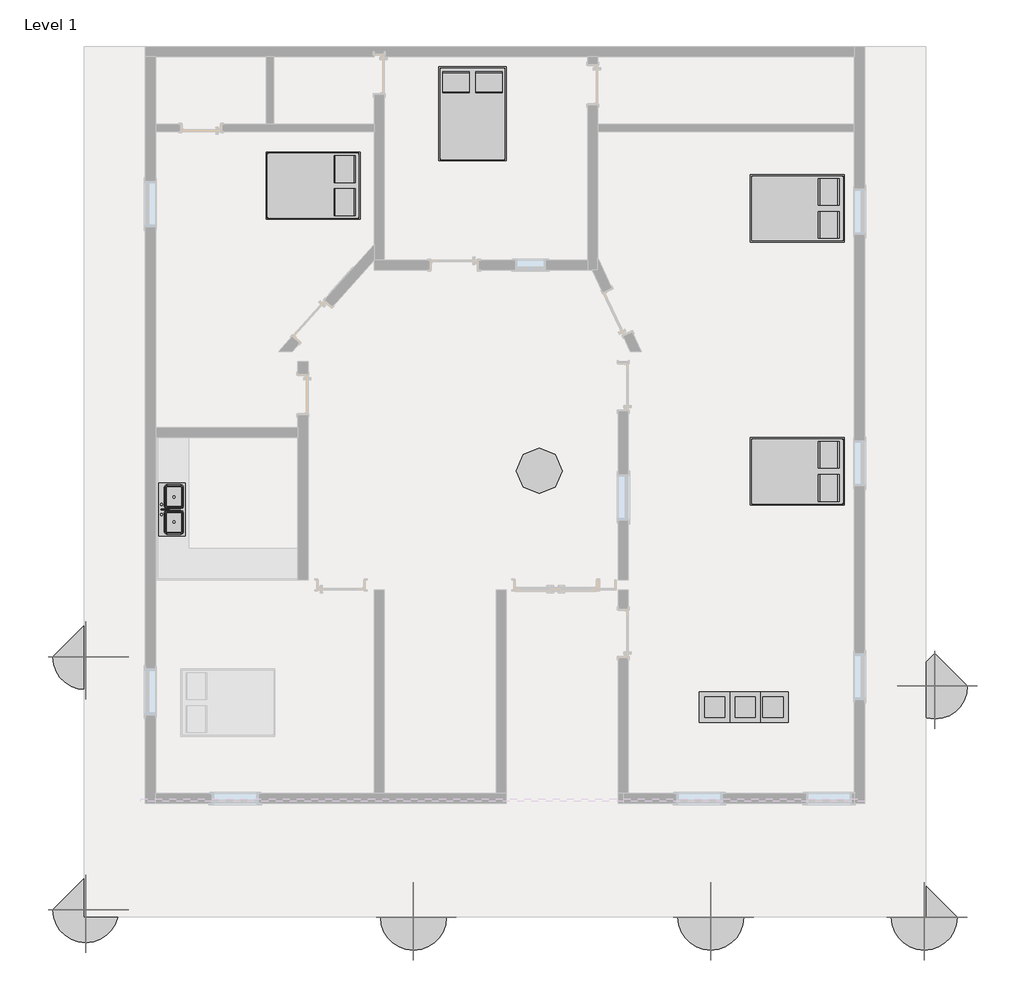
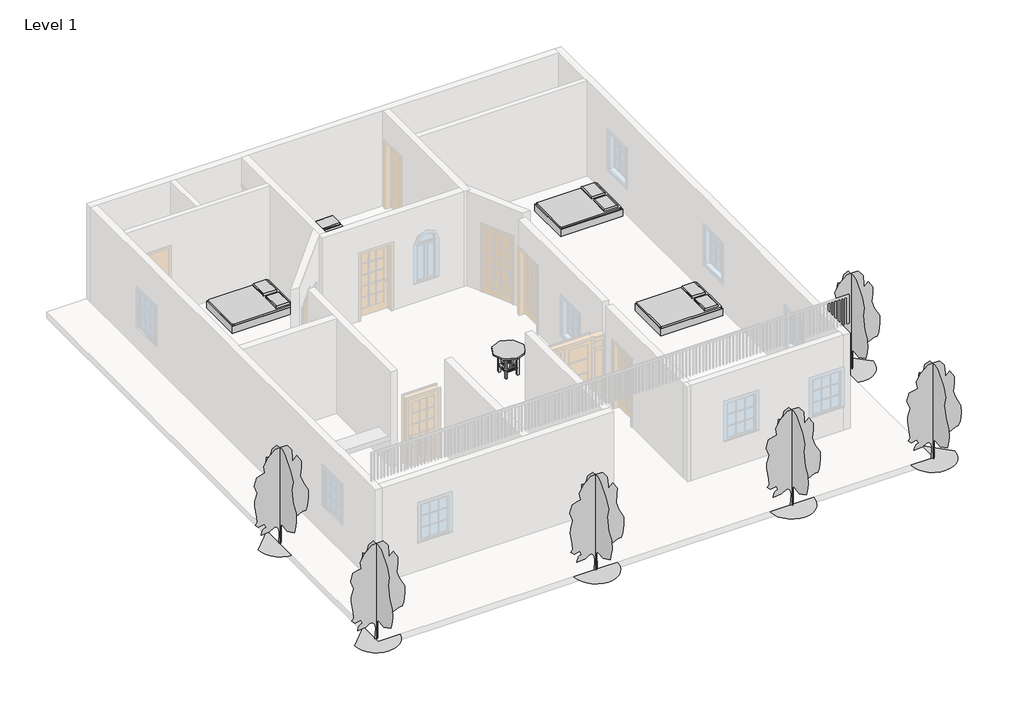
# One storey, part 3 of 3: 8 furniture elements, 6 geographic elements, 1 flow terminal.
"""IFC4 building model written with IfcOpenShell, lengths in millimetres."""

from ifc_helpers import new_model, si_unit, origin, place, context, project, spatial, transform, mapped, element, save
from components import flow_terminal_a53be723, furniture_c8abb964, furniture_b5c51a22, furniture_905aceb5, rpc_tree_deciduous_red_ash_25_5dd3353f

model = new_model("IFC4")

# Units and contexts
model_context = context("Model", 3, world=origin())
ifc_project = project(units=[si_unit("LENGTHUNIT", "METRE", prefix="MILLI")], contexts=[model_context])

# Site, building, storey
site = spatial("IfcSite", under=ifc_project)
building = spatial("IfcBuilding", under=site)
storey = spatial("IfcBuildingStorey", under=building, Name="Level 1", Elevation=0.0)

# Flow terminal
placement = place(None, origin())
flow_terminal_shape = flow_terminal_a53be723(model_context)
element("IfcFlowTerminal", 1, ObjectType="Sink Kitchen-Double : 42\" x 21\"", at=placement, inside=storey, context=model_context, shape_type="MappedRepresentation", body=[
    mapped(flow_terminal_shape, transform((-9002.3643866, 9259.041554, 0.0), x_axis=(0.0, 1.0, 0.0), y_axis=(-1.0, 0.0, 0.0), z_axis=(0.0, 0.0, 1.0))),
])

# Furniture
furniture_shape = furniture_c8abb964(model_context)
element("IfcFurniture", 2, ObjectType="Bed-Box : Double 53\" x 74\"", at=placement, inside=storey, context=model_context, shape_type="MappedRepresentation", body=[
    mapped(furniture_shape, transform((-3336.7622467, 17421.2603028, 0.0), x_axis=(1.0, 0.0, 0.0), y_axis=(0.0, 1.0, 0.0), z_axis=(0.0, 0.0, 1.0))),
])
element("IfcFurniture", 3, ObjectType="Bed-Box : Double 53\" x 74\"", at=placement, inside=storey, context=model_context, shape_type="MappedRepresentation", body=[
    mapped(furniture_shape, transform((-5950.8802795, 16090.8832536, 0.0), x_axis=(0.0, -0.9999999999999997, 0.0), y_axis=(0.9999999999999997, 0.0, 0.0), z_axis=(0.0, 0.0, 1.0))),
])
element("IfcFurniture", 4, ObjectType="Bed-Box : Double 53\" x 74\"", at=placement, inside=storey, context=model_context, shape_type="MappedRepresentation", body=[
    mapped(furniture_shape, transform((3726.5197205, 15633.6832536, 0.0), x_axis=(0.0, -1.0, 0.0), y_axis=(1.0, 0.0, 0.0), z_axis=(0.0, 0.0, 1.0))),
])
element("IfcFurniture", 5, ObjectType="Bed-Box : Double 53\" x 74\"", at=placement, inside=storey, context=model_context, shape_type="MappedRepresentation", body=[
    mapped(furniture_shape, transform((3726.5197205, 10375.8832536, 0.0), x_axis=(0.0, -1.0, 0.0), y_axis=(1.0, 0.0, 0.0), z_axis=(0.0, 0.0, 1.0))),
])
furniture_2_shape = furniture_b5c51a22(model_context)
element("IfcFurniture", 6, ObjectType="Table-Coffee : 24\" x 24\" x 24\"", at=placement, inside=storey, context=model_context, shape_type="MappedRepresentation", body=[
    mapped(furniture_2_shape, transform((2432.4244457, 5229.8197168, 0.0), x_axis=(1.0, 0.0, 0.0), y_axis=(0.0, 1.0, 0.0), z_axis=(0.0, 0.0, 1.0))),
])
element("IfcFurniture", 7, ObjectType="Table-Coffee : 24\" x 24\" x 24\"", at=placement, inside=storey, context=model_context, shape_type="MappedRepresentation", body=[
    mapped(furniture_2_shape, transform((1822.8244457, 5229.8197168, 0.0), x_axis=(1.0, 0.0, 0.0), y_axis=(0.0, 1.0, 0.0), z_axis=(0.0, 0.0, 1.0))),
])
element("IfcFurniture", 8, ObjectType="Table-Coffee : 24\" x 24\" x 24\"", at=placement, inside=storey, context=model_context, shape_type="MappedRepresentation", body=[
    mapped(furniture_2_shape, transform((2991.2244457, 5229.8197168, 0.0), x_axis=(1.0, 0.0, 0.0), y_axis=(0.0, 1.0, 0.0), z_axis=(0.0, 0.0, 1.0))),
])
furniture_3_shape = furniture_905aceb5(model_context)
element("IfcFurniture", 9, ObjectType="Table-Dining Round w Chairs : 36\" Diameter", at=placement, inside=storey, context=model_context, shape_type="MappedRepresentation", body=[
    mapped(furniture_3_shape, transform((-1767.7917549, 10234.3094831, 0.0), x_axis=(1.0, 0.0, 0.0), y_axis=(0.0, 1.0, 0.0), z_axis=(0.0, 0.0, 1.0))),
])

# Geographic elements
rpc_tree_deciduous_red_ash_25_shape = rpc_tree_deciduous_red_ash_25_5dd3353f(model_context)
element("IfcGeographicElement", 10, ObjectType="RPC Tree - Deciduous : Red Ash - 25'", at=placement, inside=storey, context=model_context, shape_type="MappedRepresentation", body=[
    mapped(rpc_tree_deciduous_red_ash_25_shape, transform((6032.0902123, 1121.3307946, 0.0), x_axis=(1.0, 0.0, 0.0), y_axis=(0.0, 1.0, 0.0), z_axis=(0.0, 0.0, 1.0))),
])
element("IfcGeographicElement", 11, ObjectType="RPC Tree - Deciduous : Red Ash - 25'", at=placement, inside=storey, context=model_context, shape_type="MappedRepresentation", body=[
    mapped(rpc_tree_deciduous_red_ash_25_shape, transform((-10731.9097877, 1273.7307946, 0.0), x_axis=(1.0, 0.0, 0.0), y_axis=(0.0, 1.0, 0.0), z_axis=(0.0, 0.0, 1.0))),
])
element("IfcGeographicElement", 12, ObjectType="RPC Tree - Deciduous : Red Ash - 25'", at=placement, inside=storey, context=model_context, shape_type="MappedRepresentation", body=[
    mapped(rpc_tree_deciduous_red_ash_25_shape, transform((-4178.7097877, 1121.3307946, 0.0), x_axis=(1.0, 0.0, 0.0), y_axis=(0.0, 1.0, 0.0), z_axis=(0.0, 0.0, 1.0))),
])
element("IfcGeographicElement", 13, ObjectType="RPC Tree - Deciduous : Red Ash - 25'", at=placement, inside=storey, context=model_context, shape_type="MappedRepresentation", body=[
    mapped(rpc_tree_deciduous_red_ash_25_shape, transform((1764.8902123, 1121.3307946, 0.0), x_axis=(1.0, 0.0, 0.0), y_axis=(0.0, 1.0, 0.0), z_axis=(0.0, 0.0, 1.0))),
])
element("IfcGeographicElement", 14, ObjectType="RPC Tree - Deciduous : Red Ash - 25'", at=placement, inside=storey, context=model_context, shape_type="MappedRepresentation", body=[
    mapped(rpc_tree_deciduous_red_ash_25_shape, transform((6235.2902123, 5744.1307946, 0.0), x_axis=(1.0, 0.0, 0.0), y_axis=(0.0, 1.0, 0.0), z_axis=(0.0, 0.0, 1.0))),
])
element("IfcGeographicElement", 15, ObjectType="RPC Tree - Deciduous : Red Ash - 25'", at=placement, inside=storey, context=model_context, shape_type="MappedRepresentation", body=[
    mapped(rpc_tree_deciduous_red_ash_25_shape, transform((-10731.9097877, 6331.3165494, 0.0), x_axis=(1.0, 0.0, 0.0), y_axis=(0.0, 1.0, 0.0), z_axis=(0.0, 0.0, 1.0))),
])

save(model, "model.ifc")

# Revit data of these elements
# Type "Sink Kitchen-Double : 42\" x 21\""
#   Assembly Code = "D2010410"
#   Counter Height = 3' - 0"
#   Depth = 1' - 9"
#   Width = 3' - 6"
#   Faucet Material = Steel, Polished
#   Sink Material = Steel, Polished
#   Default Elevation = 0
# Type "Bed-Box : Double 53\" x 74\""
#   Assembly Code = "E2020200"
#   Length = 6' - 2"
#   Width = 4' - 5"
#   Frame Material = Birch
#   Mattress Material = Linen, White
#   Default Elevation = 0
# Type "Table-Coffee : 24\" x 24\" x 24\""
#   Assembly Code = "E2020200"
#   Height = 2' - 0"
#   Length = 2' - 0"
#   Width = 2' - 0"
#   Top Material = none
#   Frame Material = none
#   Default Elevation = 0
# Type "Table-Dining Round w Chairs : 36\" Diameter"
#   Assembly Code = "E2020200"
#   Radius = 1' - 6"
#   Diameter = 3' - 0"
#   Height = 2' - 6"
#   Chairs = 4
#   Base Material = Pine
#   Top Material = Laminate, Linen, Matte
#   Default Elevation = 0
# Type "RPC Tree - Deciduous : Red Ash - 25'"
#   built-in parameter 1005198 = "{2, 15},{22, RPC-8-G3GR-497X-PHW5-6},{1, 0},{1, 0},{2, 15},{1, 8},{5, Color},{1, 0},{1, 0},{3, 0.8},{3, 0.8},{3, 0.8},{1, 8},{7, BBoxMin},{1, 0},{1, 0},{1, 0},{1, 0},{1, 0},{1, 8},{7, BBoxMax},{1, 0},{1, 0},{1, 0},{1, 0},{1, 0},{2, 11},{9, RPCTypeId},{1, 0},{1, 0},{22, RPC-8-G3GR-497X-PHW5-6},{1, 6},{14, RPCPlantHeight},{1, 0},{1, 0},{2, 25},{2, 11},{7, keyword},{1, 0},{1, 0},{34, :RPCs:Trees [General]:Geometry:RPC},{2, 11},{8, category},{1, 0},{1, 0},{15, Trees [General]},{2, 11},{12, LocalizedUID},{1, 0},{1, 0},{7, Red Ash},{2, 14},{6, Height},{1, 0},{1, 0},{2, 25},{1, 2},{16, Cast Reflections},{1, 0},{1, 0},{1, 0},{1, 2},{6, Jitter},{1, 0},{1, 0},{1, 1},{1, 2},{9, Billboard},{1, 0},{1, 0},{1, 0},{1, 2},{12, Cast Shadows},{1, 0},{1, 0},{1, 1},{1, 2},{20, Apply Filter Effects},{1, 0},{1, 0},{1, 0},{2, 11},{28, Apply Filter Effects-Text-FC},{1, 0},{1, 0},{4, None},{21, assetlibrary_base.fbx},{1, 5},"
#   built-in parameter 1005195 = "RPC-8-G3GR-497X-PHW5-6"
#   Type Comments = "Red Maple"
#   Assembly Code = "G2050500"
#   Height = 10' - 0"
#   Default Elevation = 0
# Element 1 (IfcFlowTerminal, "Sink Kitchen-Double : 42\" x 21\"")
#   Mark = "1"
#   Phase Created = New Construction
#   Materials on its faces: "Steel, Polished"
# Elements 2, 3, 4, 5 (IfcFurniture, "Bed-Box : Double 53\" x 74\"")
#   Phase Created = New Construction
#   Materials on its faces: "Birch", "Linen, White"
# Elements 6, 7, 8 (IfcFurniture, "Table-Coffee : 24\" x 24\" x 24\"")
#   Phase Created = New Construction
#   Materials on its faces: "Glass - Clear, Grey"
# Element 9 (IfcFurniture, "Table-Dining Round w Chairs : 36\" Diameter")
#   Phase Created = New Construction
#   Materials on its faces: "Pine", "Laminate, Linen, Matte"
# Elements 10, 11, 12, 13, 14, 15 (IfcGeographicElement, "RPC Tree - Deciduous : Red Ash - 25'")
#   Phase Created = New Construction
# Materials
#   "Steel, Polished": class "Metal", colour RGB 192 192 192, transparency 0, Description = "Polished steel", Cost = 0
#   "Birch": class "Wood", colour RGB 224 178 126, transparency 0, Description = "Betula Alleghaniensis", Cost = 0
#   "Linen, White": class "Textile", colour RGB 247 247 239, transparency 0, Description = "Linen, white", Cost = 0
#   "Pine": class "Wood", colour RGB 223 192 134, transparency 0, Description = "Pinus Echinata", Cost = 0
#   "Laminate, Linen, Matte": class "Plastic", colour RGB 249 239 230, transparency 0, Description = "Plastic Laminate - Linen, Matte", Cost = 0
#   "Glass - Clear, Grey": class "Glass", colour RGB 252 255 255, transparency 0.64
